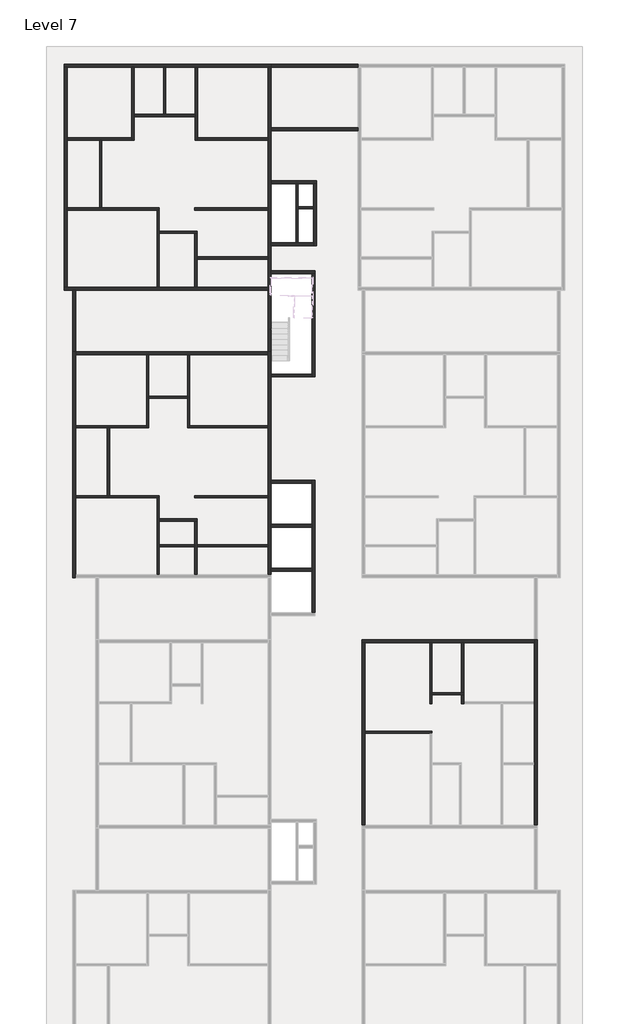
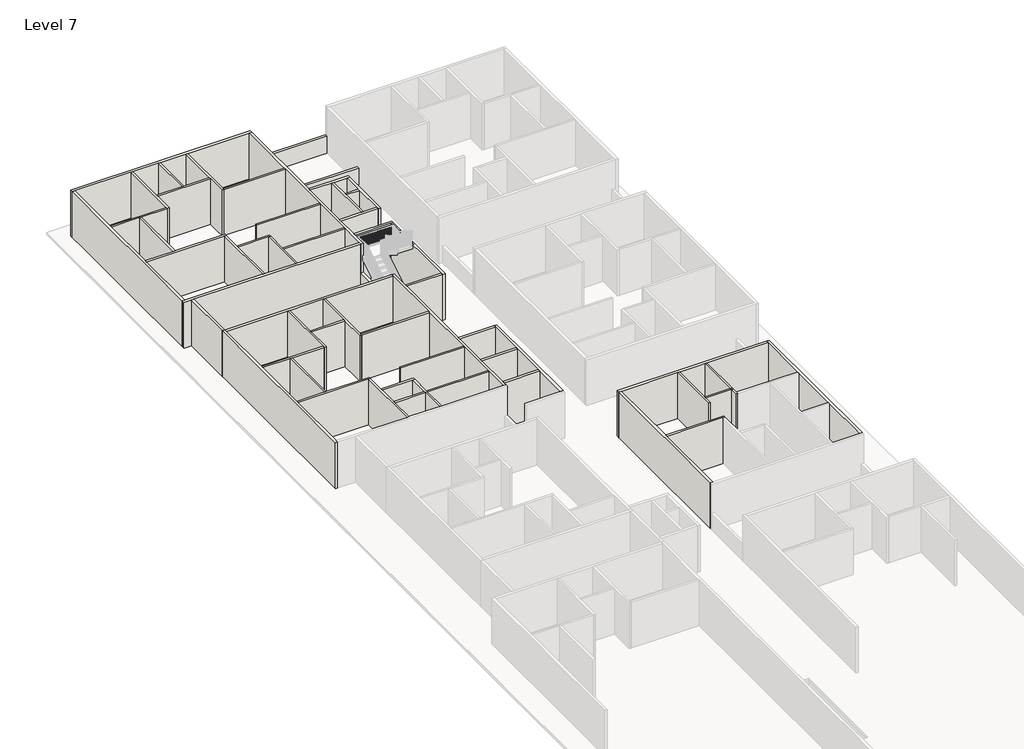
# One storey, part 3 of 8: 57 walls.
"""IFC4 building model written with IfcOpenShell, lengths in millimetres."""

from ifc_helpers import new_model, si_unit, frame, origin, place, context, project, spatial, polyline, outline, extrude, faceted_brep, element, save

model = new_model("IFC4")

# Units and contexts
model_context = context("Model", 3, world=origin())
ifc_project = project(units=[si_unit("LENGTHUNIT", "METRE", prefix="MILLI")], contexts=[model_context])

# Site, building, storey
site = spatial("IfcSite", under=ifc_project)
building = spatial("IfcBuilding", under=site)
storey = spatial("IfcBuildingStorey", under=building, Name="Level 7", Elevation=43522.6172466)

# Walls
placement = place(None, origin())
element("IfcWall", 1, ObjectType="4.5\"", at=placement, inside=storey, context=model_context, shape_type="Brep", body=[
    faceted_brep([(-10818.3415084, 35031.1216096, 43522.6172466), (-10818.3415084, 31373.5216096, 43522.6172466), (-10818.3415084, 31259.2216096, 43522.6172466), (-10818.3415084, 31259.2216096, 46570.6172466), (-10818.3415084, 31373.5216096, 46570.6172466), (-10818.3415084, 35031.1216096, 46570.6172466), (-10704.0415084, 35031.1216096, 43522.6172466), (-10704.0415084, 35031.1216096, 46570.6172466), (-10704.0415084, 32592.7216096, 46570.6172466), (-10704.0415084, 32478.4216096, 46570.6172466), (-10704.0415084, 31259.2216096, 46570.6172466), (-10704.0415084, 31259.2216096, 43522.6172466), (-10704.0415084, 32478.4216096, 43522.6172466), (-10704.0415084, 32592.7216096, 43522.6172466)], [[[0, 1, 2, 3, 4, 5]], [[6, 7, 8, 9, 10, 11, 12, 13]], [[2, 1, 0, 6, 13, 12, 11]], [[0, 5, 7, 6]], [[3, 2, 11, 10]], [[5, 4, 3, 10, 9, 8, 7]]]),
])
element("IfcWall", 2, ObjectType="4.5\"", at=placement, inside=storey, context=model_context, shape_type="Brep", body=[
    faceted_brep([(-10818.3415084, 31373.5216096, 43522.6172466), (-14171.1415084, 31373.5216096, 43522.6172466), (-14171.1415084, 31373.5216096, 46570.6172466), (-10818.3415084, 31373.5216096, 46570.6172466), (-10818.3415084, 31259.2216096, 43522.6172466), (-10818.3415084, 31259.2216096, 46570.6172466), (-12380.4415084, 31259.2216096, 46570.6172466), (-12494.7415084, 31259.2216096, 46570.6172466), (-14171.1415084, 31259.2216096, 46570.6172466), (-14171.1415084, 31259.2216096, 43522.6172466), (-12494.7415084, 31259.2216096, 43522.6172466), (-12380.4415084, 31259.2216096, 43522.6172466)], [[[0, 1, 2, 3]], [[4, 5, 6, 7, 8, 9, 10, 11]], [[1, 0, 4, 11, 10, 9]], [[0, 3, 5, 4]], [[2, 1, 9, 8]], [[3, 2, 8, 7, 6, 5]]]),
])
element("IfcWall", 3, ObjectType="4.5\"", at=placement, inside=storey, context=model_context, shape_type="SweptSolid", body=[
    extrude(outline(polyline([(-12494.7415084, 27754.0216096), (-12494.7415084, 31259.2216096), (-12380.4415084, 31259.2216096), (-12380.4415084, 27754.0216096), (-12494.7415084, 27754.0216096)])), frame((0.0, 0.0, 43522.6172466), z_axis=(0.0, 0.0, 1.0), x_axis=(1.0, 0.0, 0.0)), (0.0, 0.0, 1.0), 3048.0),
])
element("IfcWall", 4, ObjectType="4.5\"", at=placement, inside=storey, context=model_context, shape_type="Brep", body=[
    faceted_brep([(-14171.1415084, 27639.7216096, 43522.6172466), (-9510.2415084, 27639.7216096, 43522.6172466), (-9395.9415084, 27639.7216096, 43522.6172466), (-9395.9415084, 27639.7216096, 46570.6172466), (-9510.2415084, 27639.7216096, 46570.6172466), (-14171.1415084, 27639.7216096, 46570.6172466), (-14171.1415084, 27754.0216096, 43522.6172466), (-14171.1415084, 27754.0216096, 46570.6172466), (-12494.7415084, 27754.0216096, 46570.6172466), (-12380.4415084, 27754.0216096, 46570.6172466), (-9395.9415084, 27754.0216096, 46570.6172466), (-9395.9415084, 27754.0216096, 43522.6172466), (-12380.4415084, 27754.0216096, 43522.6172466), (-12494.7415084, 27754.0216096, 43522.6172466)], [[[0, 1, 2, 3, 4, 5]], [[6, 7, 8, 9, 10, 11, 12, 13]], [[2, 1, 0, 6, 13, 12, 11]], [[0, 5, 7, 6]], [[3, 2, 11, 10]], [[5, 4, 3, 10, 9, 8, 7]]]),
])
element("IfcWall", 5, ObjectType="4.5\"", at=placement, inside=storey, context=model_context, shape_type="Brep", body=[
    faceted_brep([(-9510.2415084, 27639.7216096, 43522.6172466), (-9510.2415084, 23651.9216096, 43522.6172466), (-9510.2415084, 23651.9216096, 46570.6172466), (-9510.2415084, 27639.7216096, 46570.6172466), (-9395.9415084, 27639.7216096, 43522.6172466), (-9395.9415084, 27639.7216096, 46570.6172466), (-9395.9415084, 26547.5216096, 46570.6172466), (-9395.9415084, 26433.2216096, 46570.6172466), (-9395.9415084, 23651.9216096, 46570.6172466), (-9395.9415084, 23651.9216096, 43522.6172466), (-9395.9415084, 26433.2216096, 43522.6172466), (-9395.9415084, 26547.5216096, 43522.6172466)], [[[0, 1, 2, 3]], [[4, 5, 6, 7, 8, 9, 10, 11]], [[1, 0, 4, 11, 10, 9]], [[0, 3, 5, 4]], [[2, 1, 9, 8]], [[3, 2, 8, 7, 6, 5]]]),
])
element("IfcWall", 6, ObjectType="4.5\"", at=placement, inside=storey, context=model_context, shape_type="Brep", body=[
    faceted_brep([(-9395.9415084, 26433.2216096, 43522.6172466), (-7567.1415084, 26433.2216096, 43522.6172466), (-7452.8415084, 26433.2216096, 43522.6172466), (-7452.8415084, 26433.2216096, 46570.6172466), (-7567.1415084, 26433.2216096, 46570.6172466), (-9395.9415084, 26433.2216096, 46570.6172466), (-9395.9415084, 26547.5216096, 43522.6172466), (-9395.9415084, 26547.5216096, 46570.6172466), (-7452.8415084, 26547.5216096, 46570.6172466), (-7452.8415084, 26547.5216096, 43522.6172466)], [[[0, 1, 2, 3, 4, 5]], [[6, 7, 8, 9]], [[2, 1, 0, 6, 9]], [[0, 5, 7, 6]], [[3, 2, 9, 8]], [[5, 4, 3, 8, 7]]]),
])
element("IfcWall", 7, ObjectType="4.5\"", at=placement, inside=storey, context=model_context, shape_type="Brep", body=[
    faceted_brep([(-7567.1415084, 26433.2216096, 43522.6172466), (-7567.1415084, 23651.9216096, 43522.6172466), (-7567.1415084, 23651.9216096, 46570.6172466), (-7567.1415084, 26433.2216096, 46570.6172466), (-7452.8415084, 26433.2216096, 43522.6172466), (-7452.8415084, 26433.2216096, 46570.6172466), (-7452.8415084, 25214.0216096, 46570.6172466), (-7452.8415084, 25099.7216096, 46570.6172466), (-7452.8415084, 23651.9216096, 46570.6172466), (-7452.8415084, 23651.9216096, 43522.6172466), (-7452.8415084, 25099.7216096, 43522.6172466), (-7452.8415084, 25214.0216096, 43522.6172466)], [[[0, 1, 2, 3]], [[4, 5, 6, 7, 8, 9, 10, 11]], [[1, 0, 4, 11, 10, 9]], [[0, 3, 5, 4]], [[2, 1, 9, 8]], [[3, 2, 8, 7, 6, 5]]]),
])
element("IfcWall", 8, ObjectType="4.5\"", at=placement, inside=storey, context=model_context, shape_type="SweptSolid", body=[
    extrude(outline(polyline([(-7452.8415084, 25214.0216096), (-3769.8415084, 25214.0216096), (-3769.8415084, 25099.7216096), (-7452.8415084, 25099.7216096), (-7452.8415084, 25214.0216096)])), frame((0.0, 0.0, 43522.6172466), z_axis=(0.0, 0.0, 1.0), x_axis=(1.0, 0.0, 0.0)), (0.0, 0.0, 1.0), 3048.0),
])
element("IfcWall", 9, ObjectType="4.5\"", at=placement, inside=storey, context=model_context, shape_type="SweptSolid", body=[
    extrude(outline(polyline([(-3769.8415084, 27639.7216096), (-7567.1415084, 27639.7216096), (-7567.1415084, 27754.0216096), (-3769.8415084, 27754.0216096), (-3769.8415084, 27639.7216096)])), frame((0.0, 0.0, 43522.6172466), z_axis=(0.0, 0.0, 1.0), x_axis=(1.0, 0.0, 0.0)), (0.0, 0.0, 1.0), 3048.0),
])
element("IfcWall", 10, ObjectType="4.5\"", at=placement, inside=storey, context=model_context, shape_type="Brep", body=[
    faceted_brep([(-10704.0415084, 32478.4216096, 43522.6172466), (-7541.7415084, 32478.4216096, 43522.6172466), (-7541.7415084, 32478.4216096, 46570.6172466), (-10704.0415084, 32478.4216096, 46570.6172466), (-10704.0415084, 32592.7216096, 43522.6172466), (-10704.0415084, 32592.7216096, 46570.6172466), (-9180.0415084, 32592.7216096, 46570.6172466), (-9065.7415084, 32592.7216096, 46570.6172466), (-7541.7415084, 32592.7216096, 46570.6172466), (-7541.7415084, 32592.7216096, 43522.6172466), (-9065.7415084, 32592.7216096, 43522.6172466), (-9180.0415084, 32592.7216096, 43522.6172466)], [[[0, 1, 2, 3]], [[4, 5, 6, 7, 8, 9, 10, 11]], [[1, 0, 4, 11, 10, 9]], [[0, 3, 5, 4]], [[2, 1, 9, 8]], [[3, 2, 8, 7, 6, 5]]]),
])
element("IfcWall", 11, ObjectType="4.5\"", at=placement, inside=storey, context=model_context, shape_type="SweptSolid", body=[
    extrude(outline(polyline([(-9180.0415084, 32592.7216096), (-9180.0415084, 35031.1216096), (-9065.7415084, 35031.1216096), (-9065.7415084, 32592.7216096), (-9180.0415084, 32592.7216096)])), frame((0.0, 0.0, 43522.6172466), z_axis=(0.0, 0.0, 1.0), x_axis=(1.0, 0.0, 0.0)), (0.0, 0.0, 1.0), 3048.0),
])
element("IfcWall", 12, ObjectType="4.5\"", at=placement, inside=storey, context=model_context, shape_type="Brep", body=[
    faceted_brep([(-7541.7415084, 35031.1216096, 43522.6172466), (-7541.7415084, 32592.7216096, 43522.6172466), (-7541.7415084, 32478.4216096, 43522.6172466), (-7541.7415084, 31259.2216096, 43522.6172466), (-7541.7415084, 31259.2216096, 46570.6172466), (-7541.7415084, 32478.4216096, 46570.6172466), (-7541.7415084, 32592.7216096, 46570.6172466), (-7541.7415084, 35031.1216096, 46570.6172466), (-7427.4415084, 35031.1216096, 43522.6172466), (-7427.4415084, 35031.1216096, 46570.6172466), (-7427.4415084, 31373.5216096, 46570.6172466), (-7427.4415084, 31259.2216096, 46570.6172466), (-7427.4415084, 31259.2216096, 43522.6172466), (-7427.4415084, 31373.5216096, 43522.6172466)], [[[0, 1, 2, 3, 4, 5, 6, 7]], [[8, 9, 10, 11, 12, 13]], [[3, 2, 1, 0, 8, 13, 12]], [[0, 7, 9, 8]], [[4, 3, 12, 11]], [[7, 6, 5, 4, 11, 10, 9]]]),
])
element("IfcWall", 13, ObjectType="4.5\"", at=placement, inside=storey, context=model_context, shape_type="SweptSolid", body=[
    extrude(outline(polyline([(-3769.8415084, 31259.2216096), (-7427.4415084, 31259.2216096), (-7427.4415084, 31373.5216096), (-3769.8415084, 31373.5216096), (-3769.8415084, 31259.2216096)])), frame((0.0, 0.0, 43522.6172466), z_axis=(0.0, 0.0, 1.0), x_axis=(1.0, 0.0, 0.0)), (0.0, 0.0, 1.0), 3048.0),
])
element("IfcWall", 14, ObjectType="4.5\"", at=placement, inside=storey, context=model_context, shape_type="Brep", body=[
    faceted_brep([(-10061.4044854, 20146.7216096, 43522.6172466), (-10061.4044854, 16489.1216096, 43522.6172466), (-10061.4044854, 16374.8216096, 43522.6172466), (-10061.4044854, 16374.8216096, 46570.6172466), (-10061.4044854, 16489.1216096, 46570.6172466), (-10061.4044854, 20146.7216096, 46570.6172466), (-9947.1044854, 20146.7216096, 43522.6172466), (-9947.1044854, 20146.7216096, 46570.6172466), (-9947.1044854, 18013.1216096, 46570.6172466), (-9947.1044854, 17898.8216096, 46570.6172466), (-9947.1044854, 16374.8216096, 46570.6172466), (-9947.1044854, 16374.8216096, 43522.6172466), (-9947.1044854, 17898.8216096, 43522.6172466), (-9947.1044854, 18013.1216096, 43522.6172466)], [[[0, 1, 2, 3, 4, 5]], [[6, 7, 8, 9, 10, 11, 12, 13]], [[2, 1, 0, 6, 13, 12, 11]], [[0, 5, 7, 6]], [[3, 2, 11, 10]], [[5, 4, 3, 10, 9, 8, 7]]]),
])
element("IfcWall", 15, ObjectType="4.5\"", at=placement, inside=storey, context=model_context, shape_type="Brep", body=[
    faceted_brep([(-10061.4044854, 16489.1216096, 43522.6172466), (-13719.0044854, 16489.1216096, 43522.6172466), (-13719.0044854, 16489.1216096, 46570.6172466), (-10061.4044854, 16489.1216096, 46570.6172466), (-10061.4044854, 16374.8216096, 43522.6172466), (-10061.4044854, 16374.8216096, 46570.6172466), (-11980.3915084, 16374.8216096, 46570.6172466), (-12094.6915084, 16374.8216096, 46570.6172466), (-13719.0044854, 16374.8216096, 46570.6172466), (-13719.0044854, 16374.8216096, 43522.6172466), (-12094.6915084, 16374.8216096, 43522.6172466), (-11980.3915084, 16374.8216096, 43522.6172466)], [[[0, 1, 2, 3]], [[4, 5, 6, 7, 8, 9, 10, 11]], [[1, 0, 4, 11, 10, 9]], [[0, 3, 5, 4]], [[2, 1, 9, 8]], [[3, 2, 8, 7, 6, 5]]]),
])
element("IfcWall", 16, ObjectType="4.5\"", at=placement, inside=storey, context=model_context, shape_type="SweptSolid", body=[
    extrude(outline(polyline([(-7940.5044854, 17898.8216096), (-9947.1044854, 17898.8216096), (-9947.1044854, 18013.1216096), (-7940.5044854, 18013.1216096), (-7940.5044854, 17898.8216096)])), frame((0.0, 0.0, 43522.6172466), z_axis=(0.0, 0.0, 1.0), x_axis=(1.0, 0.0, 0.0)), (0.0, 0.0, 1.0), 3048.0),
])
element("IfcWall", 17, ObjectType="4.5\"", at=placement, inside=storey, context=model_context, shape_type="Brep", body=[
    faceted_brep([(-7940.5044854, 20146.7216096, 43522.6172466), (-7940.5044854, 18013.1216096, 43522.6172466), (-7940.5044854, 17898.8216096, 43522.6172466), (-7940.5044854, 16374.8216096, 43522.6172466), (-7940.5044854, 16374.8216096, 46570.6172466), (-7940.5044854, 17898.8216096, 46570.6172466), (-7940.5044854, 18013.1216096, 46570.6172466), (-7940.5044854, 20146.7216096, 46570.6172466), (-7826.2044854, 20146.7216096, 43522.6172466), (-7826.2044854, 20146.7216096, 46570.6172466), (-7826.2044854, 16489.1216096, 46570.6172466), (-7826.2044854, 16374.8216096, 46570.6172466), (-7826.2044854, 16374.8216096, 43522.6172466), (-7826.2044854, 16489.1216096, 43522.6172466)], [[[0, 1, 2, 3, 4, 5, 6, 7]], [[8, 9, 10, 11, 12, 13]], [[3, 2, 1, 0, 8, 13, 12]], [[0, 7, 9, 8]], [[4, 3, 12, 11]], [[7, 6, 5, 4, 11, 10, 9]]]),
])
element("IfcWall", 18, ObjectType="4.5\"", at=placement, inside=storey, context=model_context, shape_type="SweptSolid", body=[
    extrude(outline(polyline([(-3769.8415084, 16374.8216096), (-7826.2044854, 16374.8216096), (-7826.2044854, 16489.1216096), (-3769.8415084, 16489.1216096), (-3769.8415084, 16374.8216096)])), frame((0.0, 0.0, 43522.6172466), z_axis=(0.0, 0.0, 1.0), x_axis=(1.0, 0.0, 0.0)), (0.0, 0.0, 1.0), 3048.0),
])
element("IfcWall", 19, ObjectType="4.5\"", at=placement, inside=storey, context=model_context, shape_type="SweptSolid", body=[
    extrude(outline(polyline([(-12094.6915084, 12869.6216096), (-12094.6915084, 16374.8216096), (-11980.3915084, 16374.8216096), (-11980.3915084, 12869.6216096), (-12094.6915084, 12869.6216096)])), frame((0.0, 0.0, 43522.6172466), z_axis=(0.0, 0.0, 1.0), x_axis=(1.0, 0.0, 0.0)), (0.0, 0.0, 1.0), 3048.0),
])
element("IfcWall", 20, ObjectType="4.5\"", at=placement, inside=storey, context=model_context, shape_type="Brep", body=[
    faceted_brep([(-13719.0044854, 12755.3216096, 43522.6172466), (-9510.2415084, 12755.3216096, 43522.6172466), (-9395.9415084, 12755.3216096, 43522.6172466), (-9395.9415084, 12755.3216096, 46570.6172466), (-9510.2415084, 12755.3216096, 46570.6172466), (-13719.0044854, 12755.3216096, 46570.6172466), (-13719.0044854, 12869.6216096, 43522.6172466), (-13719.0044854, 12869.6216096, 46570.6172466), (-12094.6915084, 12869.6216096, 46570.6172466), (-11980.3915084, 12869.6216096, 46570.6172466), (-9395.9415084, 12869.6216096, 46570.6172466), (-9395.9415084, 12869.6216096, 43522.6172466), (-11980.3915084, 12869.6216096, 43522.6172466), (-12094.6915084, 12869.6216096, 43522.6172466)], [[[0, 1, 2, 3, 4, 5]], [[6, 7, 8, 9, 10, 11, 12, 13]], [[2, 1, 0, 6, 13, 12, 11]], [[0, 5, 7, 6]], [[3, 2, 11, 10]], [[5, 4, 3, 10, 9, 8, 7]]]),
])
element("IfcWall", 21, ObjectType="4.5\"", at=placement, inside=storey, context=model_context, shape_type="Brep", body=[
    faceted_brep([(-9510.2415084, 12755.3216096, 43522.6172466), (-9510.2415084, 8767.5216096, 43522.6172466), (-9510.2415084, 8767.5216096, 46570.6172466), (-9510.2415084, 12755.3216096, 46570.6172466), (-9395.9415084, 12755.3216096, 43522.6172466), (-9395.9415084, 12755.3216096, 46570.6172466), (-9395.9415084, 11663.1216096, 46570.6172466), (-9395.9415084, 11548.8216096, 46570.6172466), (-9395.9415084, 10329.6216096, 46570.6172466), (-9395.9415084, 10215.3216096, 46570.6172466), (-9395.9415084, 8767.5216096, 46570.6172466), (-9395.9415084, 8767.5216096, 43522.6172466), (-9395.9415084, 10215.3216096, 43522.6172466), (-9395.9415084, 10329.6216096, 43522.6172466), (-9395.9415084, 11548.8216096, 43522.6172466), (-9395.9415084, 11663.1216096, 43522.6172466)], [[[0, 1, 2, 3]], [[4, 5, 6, 7, 8, 9, 10, 11, 12, 13, 14, 15]], [[1, 0, 4, 15, 14, 13, 12, 11]], [[0, 3, 5, 4]], [[2, 1, 11, 10]], [[3, 2, 10, 9, 8, 7, 6, 5]]]),
])
element("IfcWall", 22, ObjectType="4.5\"", at=placement, inside=storey, context=model_context, shape_type="SweptSolid", body=[
    extrude(outline(polyline([(-7567.1415084, 10215.3216096), (-9395.9415084, 10215.3216096), (-9395.9415084, 10329.6216096), (-7567.1415084, 10329.6216096), (-7567.1415084, 10215.3216096)])), frame((0.0, 0.0, 43522.6172466), z_axis=(0.0, 0.0, 1.0), x_axis=(1.0, 0.0, 0.0)), (0.0, 0.0, 1.0), 3048.0),
])
element("IfcWall", 23, ObjectType="4.5\"", at=placement, inside=storey, context=model_context, shape_type="Brep", body=[
    faceted_brep([(-9395.9415084, 11548.8216096, 43522.6172466), (-7567.1415084, 11548.8216096, 43522.6172466), (-7452.8415084, 11548.8216096, 43522.6172466), (-7452.8415084, 11548.8216096, 46570.6172466), (-7567.1415084, 11548.8216096, 46570.6172466), (-9395.9415084, 11548.8216096, 46570.6172466), (-9395.9415084, 11663.1216096, 43522.6172466), (-9395.9415084, 11663.1216096, 46570.6172466), (-7452.8415084, 11663.1216096, 46570.6172466), (-7452.8415084, 11663.1216096, 43522.6172466)], [[[0, 1, 2, 3, 4, 5]], [[6, 7, 8, 9]], [[2, 1, 0, 6, 9]], [[0, 5, 7, 6]], [[3, 2, 9, 8]], [[5, 4, 3, 8, 7]]]),
])
element("IfcWall", 24, ObjectType="4.5\"", at=placement, inside=storey, context=model_context, shape_type="Brep", body=[
    faceted_brep([(-7567.1415084, 11548.8216096, 43522.6172466), (-7567.1415084, 10329.6216096, 43522.6172466), (-7567.1415084, 10215.3216096, 43522.6172466), (-7567.1415084, 8767.5216096, 43522.6172466), (-7567.1415084, 8767.5216096, 46570.6172466), (-7567.1415084, 10215.3216096, 46570.6172466), (-7567.1415084, 10329.6216096, 46570.6172466), (-7567.1415084, 11548.8216096, 46570.6172466), (-7452.8415084, 11548.8216096, 43522.6172466), (-7452.8415084, 11548.8216096, 46570.6172466), (-7452.8415084, 10329.6216096, 46570.6172466), (-7452.8415084, 10215.3216096, 46570.6172466), (-7452.8415084, 8767.5216096, 46570.6172466), (-7452.8415084, 8767.5216096, 43522.6172466), (-7452.8415084, 10215.3216096, 43522.6172466), (-7452.8415084, 10329.6216096, 43522.6172466)], [[[0, 1, 2, 3, 4, 5, 6, 7]], [[8, 9, 10, 11, 12, 13, 14, 15]], [[3, 2, 1, 0, 8, 15, 14, 13]], [[0, 7, 9, 8]], [[4, 3, 13, 12]], [[7, 6, 5, 4, 12, 11, 10, 9]]]),
])
element("IfcWall", 25, ObjectType="4.5\"", at=placement, inside=storey, context=model_context, shape_type="SweptSolid", body=[
    extrude(outline(polyline([(-3769.8415084, 10215.3216096), (-7452.8415084, 10215.3216096), (-7452.8415084, 10329.6216096), (-3769.8415084, 10329.6216096), (-3769.8415084, 10215.3216096)])), frame((0.0, 0.0, 43522.6172466), z_axis=(0.0, 0.0, 1.0), x_axis=(1.0, 0.0, 0.0)), (0.0, 0.0, 1.0), 3048.0),
])
element("IfcWall", 26, ObjectType="4.5\"", at=placement, inside=storey, context=model_context, shape_type="SweptSolid", body=[
    extrude(outline(polyline([(-3769.8415084, 12755.3216096), (-7567.1415084, 12755.3216096), (-7567.1415084, 12869.6216096), (-3769.8415084, 12869.6216096), (-3769.8415084, 12755.3216096)])), frame((0.0, 0.0, 43522.6172466), z_axis=(0.0, 0.0, 1.0), x_axis=(1.0, 0.0, 0.0)), (0.0, 0.0, 1.0), 3048.0),
])
element("IfcWall", 27, ObjectType="4.5\"", at=placement, inside=storey, context=model_context, shape_type="Brep", body=[
    faceted_brep([(1259.3584916, 572.7745083, 43522.6172466), (4610.8714687, 572.7745083, 43522.6172466), (4725.1714687, 572.7745083, 43522.6172466), (4725.1714687, 572.7745083, 46570.6172466), (4610.8714687, 572.7745083, 46570.6172466), (1259.3584916, 572.7745083, 46570.6172466), (1259.3584916, 687.0745083, 43522.6172466), (1259.3584916, 687.0745083, 46570.6172466), (4725.1714687, 687.0745083, 46570.6172466), (4725.1714687, 687.0745083, 43522.6172466)], [[[0, 1, 2, 3, 4, 5]], [[6, 7, 8, 9]], [[2, 1, 0, 6, 9]], [[0, 5, 7, 6]], [[3, 2, 9, 8]], [[5, 4, 3, 8, 7]]]),
])
element("IfcWall", 28, ObjectType="4.5\"", at=placement, inside=storey, context=model_context, shape_type="Brep", body=[
    faceted_brep([(4610.8714687, 5262.3216096, 43522.6172466), (4610.8714687, 2100.0216096, 43522.6172466), (4610.8714687, 2100.0216096, 46570.6172466), (4610.8714687, 5262.3216096, 46570.6172466), (4725.1714687, 5262.3216096, 43522.6172466), (4725.1714687, 5262.3216096, 46570.6172466), (4725.1714687, 2671.5216096, 46570.6172466), (4725.1714687, 2557.2216096, 46570.6172466), (4725.1714687, 2100.0216096, 46570.6172466), (4725.1714687, 2100.0216096, 43522.6172466), (4725.1714687, 2557.2216096, 43522.6172466), (4725.1714687, 2671.5216096, 43522.6172466)], [[[0, 1, 2, 3]], [[4, 5, 6, 7, 8, 9, 10, 11]], [[1, 0, 4, 11, 10, 9]], [[2, 1, 9, 8]], [[0, 3, 5, 4]], [[3, 2, 8, 7, 6, 5]]]),
])
element("IfcWall", 29, ObjectType="4.5\"", at=placement, inside=storey, context=model_context, shape_type="Brep", body=[
    faceted_brep([(4725.1714687, 2557.2216096, 43522.6172466), (6249.1714687, 2557.2216096, 43522.6172466), (6363.4714687, 2557.2216096, 43522.6172466), (6363.4714687, 2557.2216096, 46570.6172466), (6249.1714687, 2557.2216096, 46570.6172466), (4725.1714687, 2557.2216096, 46570.6172466), (4725.1714687, 2671.5216096, 43522.6172466), (4725.1714687, 2671.5216096, 46570.6172466), (6249.1714687, 2671.5216096, 46570.6172466), (6363.4714687, 2671.5216096, 46570.6172466), (6363.4714687, 2671.5216096, 43522.6172466), (6249.1714687, 2671.5216096, 43522.6172466)], [[[0, 1, 2, 3, 4, 5]], [[6, 7, 8, 9, 10, 11]], [[2, 1, 0, 6, 11, 10]], [[0, 5, 7, 6]], [[3, 2, 10, 9]], [[5, 4, 3, 9, 8, 7]]]),
])
element("IfcWall", 30, ObjectType="4.5\"", at=placement, inside=storey, context=model_context, shape_type="SweptSolid", body=[
    extrude(outline(polyline([(6363.4714687, 5262.3216096), (6363.4714687, 2671.5216096), (6249.1714687, 2671.5216096), (6249.1714687, 5262.3216096), (6363.4714687, 5262.3216096)])), frame((0.0, 0.0, 43522.6172466), z_axis=(0.0, 0.0, 1.0), x_axis=(1.0, 0.0, 0.0)), (0.0, 0.0, 1.0), 3048.0),
])
element("IfcWall", 31, ObjectType="4.5\"", at=placement, inside=storey, context=model_context, shape_type="Brep", body=[
    faceted_brep([(6249.1714687, 2557.2216096, 43522.6172466), (6249.1714687, 2100.0216096, 43522.6172466), (6249.1714687, 2100.0216096, 46570.6172466), (6249.1714687, 2557.2216096, 46570.6172466), (6363.4714687, 2557.2216096, 43522.6172466), (6363.4714687, 2557.2216096, 46570.6172466), (6363.4714687, 2214.3216096, 46570.6172466), (6363.4714687, 2100.0216096, 46570.6172466), (6363.4714687, 2100.0216096, 43522.6172466), (6363.4714687, 2214.3216096, 43522.6172466)], [[[0, 1, 2, 3]], [[4, 5, 6, 7, 8, 9]], [[1, 0, 4, 9, 8]], [[0, 3, 5, 4]], [[2, 1, 8, 7]], [[3, 2, 7, 6, 5]]]),
])
element("IfcWall", 32, ObjectType="4.5\"", at=placement, inside=storey, context=model_context, shape_type="Brep", body=[
    faceted_brep([(-2321.9738684, 29000.0900967, 43522.6172466), (-2321.9738684, 25952.0900967, 43522.6172466), (-2321.9738684, 25952.0900967, 46570.6172466), (-2321.9738684, 29000.0900967, 46570.6172466), (-2207.6738684, 29000.0900967, 43522.6172466), (-2207.6738684, 29000.0900967, 46570.6172466), (-2207.6738684, 27820.8172885, 46570.6172466), (-2207.6738684, 27706.5172885, 46570.6172466), (-2207.6738684, 25952.0900967, 46570.6172466), (-2207.6738684, 25952.0900967, 43522.6172466), (-2207.6738684, 27706.5172885, 43522.6172466), (-2207.6738684, 27820.8172885, 43522.6172466)], [[[0, 1, 2, 3]], [[4, 5, 6, 7, 8, 9, 10, 11]], [[1, 0, 4, 11, 10, 9]], [[3, 2, 8, 7, 6, 5]], [[0, 3, 5, 4]], [[2, 1, 9, 8]]]),
])
element("IfcWall", 33, ObjectType="4.5\"", at=placement, inside=storey, context=model_context, shape_type="SweptSolid", body=[
    extrude(outline(polyline([(-2207.6738684, 27820.8172885), (-1407.6415084, 27820.8172885), (-1407.6415084, 27706.5172885), (-2207.6738684, 27706.5172885), (-2207.6738684, 27820.8172885)])), frame((0.0, 0.0, 43522.6172466), z_axis=(0.0, 0.0, 1.0), x_axis=(1.0, 0.0, 0.0)), (0.0, 0.0, 1.0), 3048.0),
])
element("IfcWall", 34, ObjectType="6\"", at=placement, inside=storey, context=model_context, shape_type="Brep", body=[
    faceted_brep([(-14323.5415084, 35031.1216096, 43522.6172466), (-14171.1415084, 35031.1216096, 43522.6172466), (-10818.3415084, 35031.1216096, 43522.6172466), (-10704.0415084, 35031.1216096, 43522.6172466), (-9180.0415084, 35031.1216096, 43522.6172466), (-9065.7415084, 35031.1216096, 43522.6172466), (-7541.7415084, 35031.1216096, 43522.6172466), (-7427.4415084, 35031.1216096, 43522.6172466), (-3769.8415084, 35031.1216096, 43522.6172466), (-3617.4415084, 35031.1216096, 43522.6172466), (-3617.4415084, 35031.1216096, 46570.6172466), (-3769.8415084, 35031.1216096, 46570.6172466), (-7427.4415084, 35031.1216096, 46570.6172466), (-7541.7415084, 35031.1216096, 46570.6172466), (-9065.7415084, 35031.1216096, 46570.6172466), (-9180.0415084, 35031.1216096, 46570.6172466), (-10704.0415084, 35031.1216096, 46570.6172466), (-10818.3415084, 35031.1216096, 46570.6172466), (-14171.1415084, 35031.1216096, 46570.6172466), (-14323.5415084, 35031.1216096, 46570.6172466), (-14323.5415084, 35183.5216096, 43522.6172466), (-14323.5415084, 35183.5216096, 46570.6172466), (-3617.4415084, 35183.5216096, 46570.6172466), (-3617.4415084, 35183.5216096, 43522.6172466)], [[[0, 1, 2, 3, 4, 5, 6, 7, 8, 9, 10, 11, 12, 13, 14, 15, 16, 17, 18, 19]], [[20, 21, 22, 23]], [[9, 8, 7, 6, 5, 4, 3, 2, 1, 0, 20, 23]], [[0, 19, 21, 20]], [[9, 23, 22, 10]], [[19, 18, 17, 16, 15, 14, 13, 12, 11, 10, 22, 21]]]),
])
element("IfcWall", 35, ObjectType="6\"", at=placement, inside=storey, context=model_context, shape_type="Brep", body=[
    faceted_brep([(-3769.8415084, 35031.1216096, 46570.6172466), (-3769.8415084, 35031.1216096, 43522.6172466), (-3769.8415084, 31373.5216096, 43522.6172466), (-3769.8415084, 31259.2216096, 43522.6172466), (-3769.8415084, 27754.0216096, 43522.6172466), (-3769.8415084, 27639.7216096, 43522.6172466), (-3769.8415084, 25214.0216096, 43522.6172466), (-3769.8415084, 25099.7216096, 43522.6172466), (-3769.8415084, 23651.9216096, 43522.6172466), (-3769.8415084, 23499.5216096, 43522.6172466), (-3769.8415084, 23499.5216096, 46570.6172466), (-3769.8415084, 23651.9216096, 46570.6172466), (-3769.8415084, 25099.7216096, 46570.6172466), (-3769.8415084, 25214.0216096, 46570.6172466), (-3769.8415084, 27639.7216096, 46570.6172466), (-3769.8415084, 27754.0216096, 46570.6172466), (-3769.8415084, 31259.2216096, 46570.6172466), (-3769.8415084, 31373.5216096, 46570.6172466), (-3617.4415084, 35031.1216096, 43522.6172466), (-3617.4415084, 35031.1216096, 46570.6172466), (-3617.4415084, 29152.4900967, 46570.6172466), (-3617.4415084, 29000.0900967, 46570.6172466), (-3617.4415084, 25952.0900967, 46570.6172466), (-3617.4415084, 25799.6900967, 46570.6172466), (-3617.4415084, 24490.1216096, 46570.6172466), (-3617.4415084, 24337.7216096, 46570.6172466), (-3617.4415084, 23499.5216096, 46570.6172466), (-3617.4415084, 23499.5216096, 43522.6172466), (-3617.4415084, 24337.7216096, 43522.6172466), (-3617.4415084, 24490.1216096, 43522.6172466), (-3617.4415084, 25799.6900967, 43522.6172466), (-3617.4415084, 25952.0900967, 43522.6172466), (-3617.4415084, 29000.0900967, 43522.6172466), (-3617.4415084, 29152.4900967, 43522.6172466), (-3617.4415084, 31744.9197155, 43522.6172466), (-3617.4415084, 31897.3197155, 43522.6172466)], [[[0, 1, 2, 3, 4, 5, 6, 7, 8, 9, 10, 11, 12, 13, 14, 15, 16, 17]], [[18, 19, 20, 21, 22, 23, 24, 25, 26, 27, 28, 29, 30, 31, 32, 33, 34, 35]], [[9, 8, 7, 6, 5, 4, 3, 2, 1, 18, 35, 34, 33, 32, 31, 30, 29, 28, 27]], [[0, 19, 18, 1]], [[9, 27, 26, 10]], [[0, 17, 16, 15, 14, 13, 12, 11, 10, 26, 25, 24, 23, 22, 21, 20, 19]]]),
])
element("IfcWall", 36, ObjectType="6\"", at=placement, inside=storey, context=model_context, shape_type="Brep", body=[
    faceted_brep([(-3769.8415084, 23651.9216096, 46570.6172466), (-3769.8415084, 23651.9216096, 43522.6172466), (-7452.8415084, 23651.9216096, 43522.6172466), (-7567.1415084, 23651.9216096, 43522.6172466), (-9395.9415084, 23651.9216096, 43522.6172466), (-9510.2415084, 23651.9216096, 43522.6172466), (-14171.1415084, 23651.9216096, 43522.6172466), (-14323.5415084, 23651.9216096, 43522.6172466), (-14323.5415084, 23651.9216096, 46570.6172466), (-14171.1415084, 23651.9216096, 46570.6172466), (-9510.2415084, 23651.9216096, 46570.6172466), (-9395.9415084, 23651.9216096, 46570.6172466), (-7567.1415084, 23651.9216096, 46570.6172466), (-7452.8415084, 23651.9216096, 46570.6172466), (-3769.8415084, 23499.5216096, 43522.6172466), (-3769.8415084, 23499.5216096, 46570.6172466), (-13719.0044854, 23499.5216096, 46570.6172466), (-13871.4044854, 23499.5216096, 46570.6172466), (-14323.5415084, 23499.5216096, 46570.6172466), (-14323.5415084, 23499.5216096, 43522.6172466), (-13871.4044854, 23499.5216096, 43522.6172466), (-13719.0044854, 23499.5216096, 43522.6172466)], [[[0, 1, 2, 3, 4, 5, 6, 7, 8, 9, 10, 11, 12, 13]], [[14, 15, 16, 17, 18, 19, 20, 21]], [[7, 6, 5, 4, 3, 2, 1, 14, 21, 20, 19]], [[8, 7, 19, 18]], [[0, 15, 14, 1]], [[0, 13, 12, 11, 10, 9, 8, 18, 17, 16, 15]]]),
])
element("IfcWall", 37, ObjectType="6\"", at=placement, inside=storey, context=model_context, shape_type="Brep", body=[
    faceted_brep([(-14171.1415084, 23651.9216096, 43522.6172466), (-14171.1415084, 27639.7216096, 43522.6172466), (-14171.1415084, 27754.0216096, 43522.6172466), (-14171.1415084, 31259.2216096, 43522.6172466), (-14171.1415084, 31373.5216096, 43522.6172466), (-14171.1415084, 35031.1216096, 43522.6172466), (-14171.1415084, 35031.1216096, 46570.6172466), (-14171.1415084, 31373.5216096, 46570.6172466), (-14171.1415084, 31259.2216096, 46570.6172466), (-14171.1415084, 27754.0216096, 46570.6172466), (-14171.1415084, 27639.7216096, 46570.6172466), (-14171.1415084, 23651.9216096, 46570.6172466), (-14323.5415084, 23651.9216096, 43522.6172466), (-14323.5415084, 23651.9216096, 46570.6172466), (-14323.5415084, 35031.1216096, 46570.6172466), (-14323.5415084, 35031.1216096, 43522.6172466)], [[[0, 1, 2, 3, 4, 5, 6, 7, 8, 9, 10, 11]], [[12, 13, 14, 15]], [[5, 4, 3, 2, 1, 0, 12, 15]], [[6, 5, 15, 14]], [[0, 11, 13, 12]], [[11, 10, 9, 8, 7, 6, 14, 13]]]),
])
element("IfcWall", 38, ObjectType="6\"", at=placement, inside=storey, context=model_context, shape_type="Brep", body=[
    faceted_brep([(-13871.4044854, 20299.1216096, 43522.6172466), (-13871.4044854, 8615.1216096, 43522.6172466), (-13871.4044854, 8615.1216096, 46570.6172466), (-13871.4044854, 20299.1216096, 46570.6172466), (-13719.0044854, 20299.1216096, 43522.6172466), (-13719.0044854, 20299.1216096, 46570.6172466), (-13719.0044854, 20146.7216096, 46570.6172466), (-13719.0044854, 16489.1216096, 46570.6172466), (-13719.0044854, 16374.8216096, 46570.6172466), (-13719.0044854, 12869.6216096, 46570.6172466), (-13719.0044854, 12755.3216096, 46570.6172466), (-13719.0044854, 8767.5216096, 46570.6172466), (-13719.0044854, 8615.1216096, 46570.6172466), (-13719.0044854, 8615.1216096, 43522.6172466), (-13719.0044854, 8767.5216096, 43522.6172466), (-13719.0044854, 12755.3216096, 43522.6172466), (-13719.0044854, 12869.6216096, 43522.6172466), (-13719.0044854, 16374.8216096, 43522.6172466), (-13719.0044854, 16489.1216096, 43522.6172466), (-13719.0044854, 20146.7216096, 43522.6172466)], [[[0, 1, 2, 3]], [[4, 5, 6, 7, 8, 9, 10, 11, 12, 13, 14, 15, 16, 17, 18, 19]], [[1, 0, 4, 19, 18, 17, 16, 15, 14, 13]], [[2, 1, 13, 12]], [[0, 3, 5, 4]], [[3, 2, 12, 11, 10, 9, 8, 7, 6, 5]]]),
])
element("IfcWall", 39, ObjectType="6\"", at=placement, inside=storey, context=model_context, shape_type="Brep", body=[
    faceted_brep([(-3617.4415084, 8767.5216096, 46570.6172466), (-3617.4415084, 8767.5216096, 43522.6172466), (-3617.4415084, 8945.2303368, 43522.6172466), (-3617.4415084, 9097.6303368, 43522.6172466), (-3617.4415084, 11231.2303368, 43522.6172466), (-3617.4415084, 11383.6303368, 43522.6172466), (-3617.4415084, 13517.2303368, 43522.6172466), (-3617.4415084, 13669.6303368, 43522.6172466), (-3617.4415084, 19003.7216096, 43522.6172466), (-3617.4415084, 19156.1216096, 43522.6172466), (-3617.4415084, 20299.1216096, 43522.6172466), (-3617.4415084, 20299.1216096, 46570.6172466), (-3617.4415084, 19156.1216096, 46570.6172466), (-3617.4415084, 19003.7216096, 46570.6172466), (-3617.4415084, 13669.6303368, 46570.6172466), (-3617.4415084, 13517.2303368, 46570.6172466), (-3617.4415084, 11383.6303368, 46570.6172466), (-3617.4415084, 11231.2303368, 46570.6172466), (-3617.4415084, 9097.6303368, 46570.6172466), (-3617.4415084, 8945.2303368, 46570.6172466), (-3769.8415084, 8767.5216096, 43522.6172466), (-3769.8415084, 8767.5216096, 46570.6172466), (-3769.8415084, 10215.3216096, 46570.6172466), (-3769.8415084, 10329.6216096, 46570.6172466), (-3769.8415084, 12755.3216096, 46570.6172466), (-3769.8415084, 12869.6216096, 46570.6172466), (-3769.8415084, 16374.8216096, 46570.6172466), (-3769.8415084, 16489.1216096, 46570.6172466), (-3769.8415084, 20146.7216096, 46570.6172466), (-3769.8415084, 20299.1216096, 46570.6172466), (-3769.8415084, 20299.1216096, 43522.6172466), (-3769.8415084, 20146.7216096, 43522.6172466), (-3769.8415084, 16489.1216096, 43522.6172466), (-3769.8415084, 16374.8216096, 43522.6172466), (-3769.8415084, 12869.6216096, 43522.6172466), (-3769.8415084, 12755.3216096, 43522.6172466), (-3769.8415084, 10329.6216096, 43522.6172466), (-3769.8415084, 10215.3216096, 43522.6172466)], [[[0, 1, 2, 3, 4, 5, 6, 7, 8, 9, 10, 11, 12, 13, 14, 15, 16, 17, 18, 19]], [[20, 21, 22, 23, 24, 25, 26, 27, 28, 29, 30, 31, 32, 33, 34, 35, 36, 37]], [[10, 9, 8, 7, 6, 5, 4, 3, 2, 1, 20, 37, 36, 35, 34, 33, 32, 31, 30]], [[10, 30, 29, 11]], [[0, 21, 20, 1]], [[0, 19, 18, 17, 16, 15, 14, 13, 12, 11, 29, 28, 27, 26, 25, 24, 23, 22, 21]]]),
])
element("IfcWall", 40, ObjectType="6\"", at=placement, inside=storey, context=model_context, shape_type="Brep", body=[
    faceted_brep([(-3769.8415084, 20299.1216096, 46570.6172466), (-3769.8415084, 20299.1216096, 43522.6172466), (-13719.0044854, 20299.1216096, 43522.6172466), (-13719.0044854, 20299.1216096, 46570.6172466), (-3769.8415084, 20146.7216096, 43522.6172466), (-3769.8415084, 20146.7216096, 46570.6172466), (-7826.2044854, 20146.7216096, 46570.6172466), (-7940.5044854, 20146.7216096, 46570.6172466), (-9947.1044854, 20146.7216096, 46570.6172466), (-10061.4044854, 20146.7216096, 46570.6172466), (-13719.0044854, 20146.7216096, 46570.6172466), (-13719.0044854, 20146.7216096, 43522.6172466), (-10061.4044854, 20146.7216096, 43522.6172466), (-9947.1044854, 20146.7216096, 43522.6172466), (-7940.5044854, 20146.7216096, 43522.6172466), (-7826.2044854, 20146.7216096, 43522.6172466)], [[[0, 1, 2, 3]], [[4, 5, 6, 7, 8, 9, 10, 11, 12, 13, 14, 15]], [[2, 1, 4, 15, 14, 13, 12, 11]], [[3, 2, 11, 10]], [[0, 5, 4, 1]], [[0, 3, 10, 9, 8, 7, 6, 5]]]),
])
element("IfcWall", 41, ObjectType="6\"", at=placement, inside=storey, context=model_context, shape_type="Brep", body=[
    faceted_brep([(10173.4714687, -4185.9344126, 46570.6172466), (10173.4714687, -4185.9344126, 43522.6172466), (10173.4714687, 5414.7216096, 43522.6172466), (10173.4714687, 5414.7216096, 46570.6172466), (10021.0714687, -4185.9344126, 43522.6172466), (10021.0714687, -4185.9344126, 46570.6172466), (10021.0714687, -1061.7344126, 46570.6172466), (10021.0714687, -947.4344126, 46570.6172466), (10021.0714687, 2100.0216096, 46570.6172466), (10021.0714687, 2214.3216096, 46570.6172466), (10021.0714687, 5262.3216096, 46570.6172466), (10021.0714687, 5414.7216096, 46570.6172466), (10021.0714687, 5414.7216096, 43522.6172466), (10021.0714687, 5262.3216096, 43522.6172466), (10021.0714687, 2214.3216096, 43522.6172466), (10021.0714687, 2100.0216096, 43522.6172466), (10021.0714687, -947.4344126, 43522.6172466), (10021.0714687, -1061.7344126, 43522.6172466)], [[[0, 1, 2, 3]], [[4, 5, 6, 7, 8, 9, 10, 11, 12, 13, 14, 15, 16, 17]], [[2, 1, 4, 17, 16, 15, 14, 13, 12]], [[2, 12, 11, 3]], [[0, 5, 4, 1]], [[0, 3, 11, 10, 9, 8, 7, 6, 5]]]),
])
element("IfcWall", 42, ObjectType="6\"", at=placement, inside=storey, context=model_context, shape_type="Brep", body=[
    faceted_brep([(10021.0714687, 5414.7216096, 46570.6172466), (10021.0714687, 5414.7216096, 43522.6172466), (1106.9584916, 5414.7216096, 43522.6172466), (1106.9584916, 5414.7216096, 46570.6172466), (10021.0714687, 5262.3216096, 43522.6172466), (10021.0714687, 5262.3216096, 46570.6172466), (6363.4714687, 5262.3216096, 46570.6172466), (6249.1714687, 5262.3216096, 46570.6172466), (4725.1714687, 5262.3216096, 46570.6172466), (4610.8714687, 5262.3216096, 46570.6172466), (1259.3584916, 5262.3216096, 46570.6172466), (1106.9584916, 5262.3216096, 46570.6172466), (1106.9584916, 5262.3216096, 43522.6172466), (1259.3584916, 5262.3216096, 43522.6172466), (4610.8714687, 5262.3216096, 43522.6172466), (4725.1714687, 5262.3216096, 43522.6172466), (6249.1714687, 5262.3216096, 43522.6172466), (6363.4714687, 5262.3216096, 43522.6172466)], [[[0, 1, 2, 3]], [[4, 5, 6, 7, 8, 9, 10, 11, 12, 13, 14, 15, 16, 17]], [[2, 1, 4, 17, 16, 15, 14, 13, 12]], [[3, 2, 12, 11]], [[0, 5, 4, 1]], [[0, 3, 11, 10, 9, 8, 7, 6, 5]]]),
])
element("IfcWall", 43, ObjectType="6\"", at=placement, inside=storey, context=model_context, shape_type="Brep", body=[
    faceted_brep([(1106.9584916, 5262.3216096, 43522.6172466), (1106.9584916, -4185.9344126, 43522.6172466), (1106.9584916, -4185.9344126, 46570.6172466), (1106.9584916, 5262.3216096, 46570.6172466), (1259.3584916, 5262.3216096, 43522.6172466), (1259.3584916, 5262.3216096, 46570.6172466), (1259.3584916, 687.0745083, 46570.6172466), (1259.3584916, 572.7745083, 46570.6172466), (1259.3584916, -4185.9344126, 46570.6172466), (1259.3584916, -4185.9344126, 43522.6172466), (1259.3584916, 572.7745083, 43522.6172466), (1259.3584916, 687.0745083, 43522.6172466)], [[[0, 1, 2, 3]], [[4, 5, 6, 7, 8, 9, 10, 11]], [[1, 0, 4, 11, 10, 9]], [[0, 3, 5, 4]], [[1, 9, 8, 2]], [[3, 2, 8, 7, 6, 5]]]),
])
element("IfcWall", 44, ObjectType="6\"", at=placement, inside=storey, context=model_context, shape_type="Brep", body=[
    faceted_brep([(-1331.4415084, 6811.6303368, 43522.6172466), (-1331.4415084, 13669.6303368, 43522.6172466), (-1331.4415084, 13669.6303368, 46570.6172466), (-1331.4415084, 6811.6303368, 46570.6172466), (-1483.8415084, 6811.6303368, 43522.6172466), (-1483.8415084, 6811.6303368, 46570.6172466), (-1483.8415084, 8945.2303368, 46570.6172466), (-1483.8415084, 9097.6303368, 46570.6172466), (-1483.8415084, 11231.2303368, 46570.6172466), (-1483.8415084, 11383.6303368, 46570.6172466), (-1483.8415084, 13517.2303368, 46570.6172466), (-1483.8415084, 13669.6303368, 46570.6172466), (-1483.8415084, 13669.6303368, 43522.6172466), (-1483.8415084, 13517.2303368, 43522.6172466), (-1483.8415084, 11383.6303368, 43522.6172466), (-1483.8415084, 11231.2303368, 43522.6172466), (-1483.8415084, 9097.6303368, 43522.6172466), (-1483.8415084, 8945.2303368, 43522.6172466)], [[[0, 1, 2, 3]], [[4, 5, 6, 7, 8, 9, 10, 11, 12, 13, 14, 15, 16, 17]], [[1, 0, 4, 17, 16, 15, 14, 13, 12]], [[3, 2, 11, 10, 9, 8, 7, 6, 5]], [[0, 3, 5, 4]], [[2, 1, 12, 11]]]),
])
element("IfcWall", 45, ObjectType="6\"", at=placement, inside=storey, context=model_context, shape_type="SweptSolid", body=[
    extrude(outline(polyline([(-3617.4415084, 13669.6303368), (-1483.8415084, 13669.6303368), (-1483.8415084, 13517.2303368), (-3617.4415084, 13517.2303368), (-3617.4415084, 13669.6303368)])), frame((0.0, 0.0, 43522.6172466), z_axis=(0.0, 0.0, 1.0), x_axis=(1.0, 0.0, 0.0)), (0.0, 0.0, 1.0), 3048.0),
])
element("IfcWall", 46, ObjectType="6\"", at=placement, inside=storey, context=model_context, shape_type="SweptSolid", body=[
    extrude(outline(polyline([(-1483.8415084, 8945.2303368), (-3617.4415084, 8945.2303368), (-3617.4415084, 9097.6303368), (-1483.8415084, 9097.6303368), (-1483.8415084, 8945.2303368)])), frame((0.0, 0.0, 43522.6172466), z_axis=(0.0, 0.0, 1.0), x_axis=(1.0, 0.0, 0.0)), (0.0, 0.0, 1.0), 3048.0),
])
element("IfcWall", 47, ObjectType="6\"", at=placement, inside=storey, context=model_context, shape_type="SweptSolid", body=[
    extrude(outline(polyline([(-3617.4415084, 11383.6303368), (-1483.8415084, 11383.6303368), (-1483.8415084, 11231.2303368), (-3617.4415084, 11231.2303368), (-3617.4415084, 11383.6303368)])), frame((0.0, 0.0, 43522.6172466), z_axis=(0.0, 0.0, 1.0), x_axis=(1.0, 0.0, 0.0)), (0.0, 0.0, 1.0), 3048.0),
])
element("IfcWall", 48, ObjectType="6\"", at=placement, inside=storey, context=model_context, shape_type="Brep", body=[
    faceted_brep([(-3617.4415084, 29000.0900967, 43522.6172466), (-2321.9738684, 29000.0900967, 43522.6172466), (-2207.6738684, 29000.0900967, 43522.6172466), (-1407.6415084, 29000.0900967, 43522.6172466), (-1255.2415084, 29000.0900967, 43522.6172466), (-1255.2415084, 29000.0900967, 46570.6172466), (-1407.6415084, 29000.0900967, 46570.6172466), (-2207.6738684, 29000.0900967, 46570.6172466), (-2321.9738684, 29000.0900967, 46570.6172466), (-3617.4415084, 29000.0900967, 46570.6172466), (-3617.4415084, 29152.4900967, 43522.6172466), (-3617.4415084, 29152.4900967, 46570.6172466), (-1255.2415084, 29152.4900967, 46570.6172466), (-1255.2415084, 29152.4900967, 43522.6172466)], [[[0, 1, 2, 3, 4, 5, 6, 7, 8, 9]], [[10, 11, 12, 13]], [[4, 3, 2, 1, 0, 10, 13]], [[9, 8, 7, 6, 5, 12, 11]], [[0, 9, 11, 10]], [[5, 4, 13, 12]]]),
])
element("IfcWall", 49, ObjectType="6\"", at=placement, inside=storey, context=model_context, shape_type="Brep", body=[
    faceted_brep([(-1407.6415084, 29000.0900967, 43522.6172466), (-1407.6415084, 27820.8172885, 43522.6172466), (-1407.6415084, 27706.5172885, 43522.6172466), (-1407.6415084, 25952.0900967, 43522.6172466), (-1407.6415084, 25799.6900967, 43522.6172466), (-1407.6415084, 25799.6900967, 46570.6172466), (-1407.6415084, 25952.0900967, 46570.6172466), (-1407.6415084, 27706.5172885, 46570.6172466), (-1407.6415084, 27820.8172885, 46570.6172466), (-1407.6415084, 29000.0900967, 46570.6172466), (-1255.2415084, 29000.0900967, 43522.6172466), (-1255.2415084, 29000.0900967, 46570.6172466), (-1255.2415084, 25799.6900967, 46570.6172466), (-1255.2415084, 25799.6900967, 43522.6172466)], [[[0, 1, 2, 3, 4, 5, 6, 7, 8, 9]], [[10, 11, 12, 13]], [[4, 3, 2, 1, 0, 10, 13]], [[9, 8, 7, 6, 5, 12, 11]], [[0, 9, 11, 10]], [[5, 4, 13, 12]]]),
])
element("IfcWall", 50, ObjectType="6\"", at=placement, inside=storey, context=model_context, shape_type="Brep", body=[
    faceted_brep([(-1407.6415084, 25952.0900967, 43522.6172466), (-2207.6738684, 25952.0900967, 43522.6172466), (-2321.9738684, 25952.0900967, 43522.6172466), (-3617.4415084, 25952.0900967, 43522.6172466), (-3617.4415084, 25952.0900967, 46570.6172466), (-2321.9738684, 25952.0900967, 46570.6172466), (-2207.6738684, 25952.0900967, 46570.6172466), (-1407.6415084, 25952.0900967, 46570.6172466), (-1407.6415084, 25799.6900967, 43522.6172466), (-1407.6415084, 25799.6900967, 46570.6172466), (-3617.4415084, 25799.6900967, 46570.6172466), (-3617.4415084, 25799.6900967, 43522.6172466)], [[[0, 1, 2, 3, 4, 5, 6, 7]], [[8, 9, 10, 11]], [[3, 2, 1, 0, 8, 11]], [[7, 6, 5, 4, 10, 9]], [[0, 7, 9, 8]], [[4, 3, 11, 10]]]),
])
element("IfcWall", 51, ObjectType="6\"", at=placement, inside=storey, context=model_context, shape_type="Brep", body=[
    faceted_brep([(-3617.4415084, 24337.7216096, 43522.6172466), (-1483.8415084, 24337.7216096, 43522.6172466), (-1331.4415084, 24337.7216096, 43522.6172466), (-1331.4415084, 24337.7216096, 46570.6172466), (-1483.8415084, 24337.7216096, 46570.6172466), (-3617.4415084, 24337.7216096, 46570.6172466), (-3617.4415084, 24490.1216096, 43522.6172466), (-3617.4415084, 24490.1216096, 46570.6172466), (-1331.4415084, 24490.1216096, 46570.6172466), (-1331.4415084, 24490.1216096, 43522.6172466)], [[[0, 1, 2, 3, 4, 5]], [[6, 7, 8, 9]], [[2, 1, 0, 6, 9]], [[5, 4, 3, 8, 7]], [[0, 5, 7, 6]], [[3, 2, 9, 8]]]),
])
element("IfcWall", 52, ObjectType="6\"", at=placement, inside=storey, context=model_context, shape_type="Brep", body=[
    faceted_brep([(-1483.8415084, 24337.7216096, 43522.6172466), (-1483.8415084, 19156.1216096, 43522.6172466), (-1483.8415084, 19003.7216096, 43522.6172466), (-1483.8415084, 19003.7216096, 46570.6172466), (-1483.8415084, 19156.1216096, 46570.6172466), (-1483.8415084, 24337.7216096, 46570.6172466), (-1331.4415084, 24337.7216096, 43522.6172466), (-1331.4415084, 24337.7216096, 46570.6172466), (-1331.4415084, 19003.7216096, 46570.6172466), (-1331.4415084, 19003.7216096, 43522.6172466)], [[[0, 1, 2, 3, 4, 5]], [[6, 7, 8, 9]], [[2, 1, 0, 6, 9]], [[5, 4, 3, 8, 7]], [[0, 5, 7, 6]], [[3, 2, 9, 8]]]),
])
element("IfcWall", 53, ObjectType="6\"", at=placement, inside=storey, context=model_context, shape_type="SweptSolid", body=[
    extrude(outline(polyline([(-3617.4415084, 19156.1216096), (-1483.8415084, 19156.1216096), (-1483.8415084, 19003.7216096), (-3617.4415084, 19003.7216096), (-3617.4415084, 19156.1216096)])), frame((0.0, 0.0, 43522.6172466), z_axis=(0.0, 0.0, 1.0), x_axis=(1.0, 0.0, 0.0)), (0.0, 0.0, 1.0), 3048.0),
])
element("IfcWall", 54, ObjectType="6\" 2", at=placement, inside=storey, context=model_context, shape_type="SweptSolid", body=[
    extrude(outline(polyline([(-13871.4044854, 20299.1216096), (-13871.4044854, 23499.5216096), (-13719.0044854, 23499.5216096), (-13719.0044854, 20299.1216096), (-13871.4044854, 20299.1216096)])), frame((0.0, 0.0, 43522.6172466), z_axis=(0.0, 0.0, 1.0), x_axis=(1.0, 0.0, 0.0)), (0.0, 0.0, 1.0), 3048.0),
])
element("IfcWall", 55, ObjectType="6\" 2", at=placement, inside=storey, context=model_context, shape_type="SweptSolid", body=[
    extrude(outline(polyline([(878.4443719, 35031.1216096), (-3617.4415084, 35031.1216096), (-3617.4415084, 35183.5216096), (878.4443719, 35183.5216096), (878.4443719, 35031.1216096)])), frame((0.0, 0.0, 43522.6172466), z_axis=(0.0, 0.0, 1.0), x_axis=(1.0, 0.0, 0.0)), (0.0, 0.0, 1.0), 1219.2),
])
element("IfcWall", 56, ObjectType="6\" 2", at=placement, inside=storey, context=model_context, shape_type="SweptSolid", body=[
    extrude(outline(polyline([(878.4443719, 31744.9197155), (-3617.4415084, 31744.9197155), (-3617.4415084, 31897.3197155), (878.4443719, 31897.3197155), (878.4443719, 31744.9197155)])), frame((0.0, 0.0, 43522.6172466), z_axis=(0.0, 0.0, 1.0), x_axis=(1.0, 0.0, 0.0)), (0.0, 0.0, 1.0), 1219.2),
])
element("IfcWall", 57, ObjectType="6\" 2", at=placement, inside=storey, context=model_context, shape_type="SweptSolid", body=[
    extrude(outline(polyline([(-3769.8415084, 20299.1216096), (-3769.8415084, 23499.5216096), (-3617.4415084, 23499.5216096), (-3617.4415084, 20299.1216096), (-3769.8415084, 20299.1216096)])), frame((0.0, 0.0, 43522.6172466), z_axis=(0.0, 0.0, 1.0), x_axis=(1.0, 0.0, 0.0)), (0.0, 0.0, 1.0), 1219.2),
])

save(model, "model.ifc")

# Revit data of these elements
# Type "4.5\""
#   Assembly Code = "B2010"
#   Layers, outside or top first: 0' - 4 1/2" "WALLS" (function 1)
# Type "6\""
#   Assembly Code = "B2010"
#   Layers, outside or top first: 0' - 6" "WALLS" (function 1)
# Type "6\" 2"
#   Assembly Code = "B2010"
#   Layers, outside or top first: 0' - 6" "4'" (function 1)
# Elements 1, 2, 3, 4, 5, 6, 7, 8, 9, 10, 11, 12, 13, 14, 15, 16, 17, 18, 19, 20, 21, 22, 23, 24, 25, 26, 27, 28, 29, 30, 31, 32, 33 (IfcWall, "4.5\"")
#   Top Offset = 0' - 0"
#   Base Offset = 0' - 0"
#   Unconnected Height = 10' - 0"
#   wall height = 10' - 0"
#   Phase Created = New Construction
#   Base Constraint = Level 7
#   Materials on its faces: "WALLS"
# Elements 34, 35, 36, 37, 38, 39, 40, 41, 42, 43, 44, 45, 46, 47, 48, 49, 50, 51, 52, 53 (IfcWall, "6\"")
#   Top Offset = 0' - 0"
#   Base Offset = 0' - 0"
#   Unconnected Height = 10' - 0"
#   wall height = 10' - 0"
#   Phase Created = New Construction
#   Base Constraint = Level 7
#   Materials on its faces: "WALLS"
# Element 54 (IfcWall, "6\" 2")
#   Top Offset = 0' - 0"
#   Base Offset = 0' - 0"
#   Unconnected Height = 10' - 0"
#   wall height = 10' - 0"
#   Phase Created = New Construction
#   Base Constraint = Level 7
#   Materials on its faces: "4'"
# Elements 55, 56, 57 (IfcWall, "6\" 2")
#   Top Offset = 0' - 0"
#   Base Offset = 0' - 0"
#   Unconnected Height = 4' - 0"
#   wall height = 4' - 0"
#   Phase Created = New Construction
#   Base Constraint = Level 7
#   Materials on its faces: "4'"
# Materials
#   "WALLS": class "Generic", colour RGB 120 120 120, transparency 0, Cost = 0
#   "4'": class "Generic", colour RGB 120 120 120, transparency 0, Cost = 0
